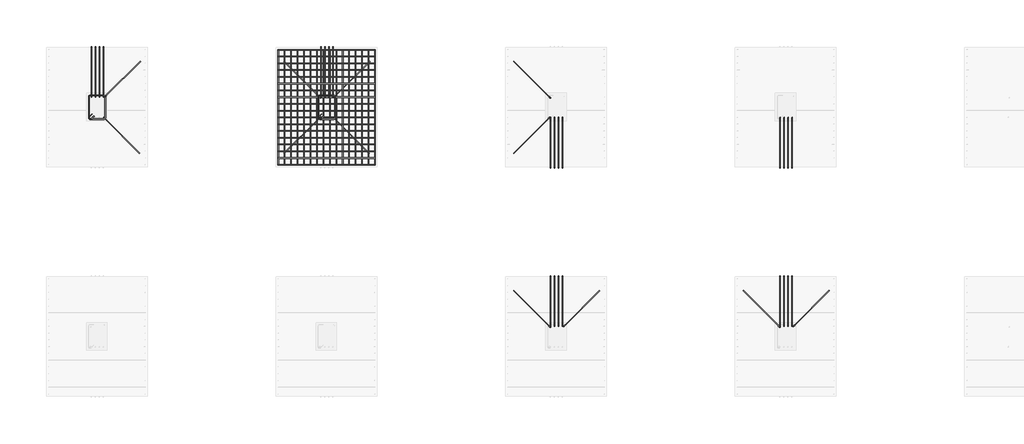
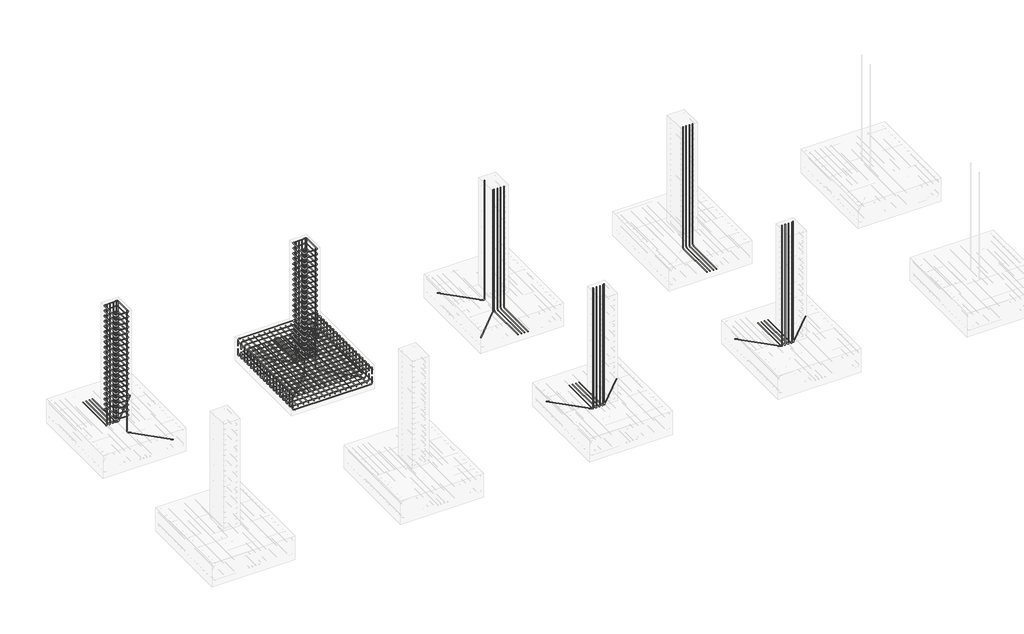
# One storey, part 9 of 33: 24 reinforcing bars.
"""IFC4 building model written with IfcOpenShell, lengths in millimetres."""

from ifc_helpers import new_model, si_unit, point, frame, origin, place, context, project, spatial, polyline, circle_curve, trimmed, segment, composite_curve, source, transform, mapped, element, save
from ifc_brep_helpers import swept_disk

model = new_model("IFC4")

# Units and contexts
model_context = context("Model", 3, world=origin())
ifc_project = project(units=[si_unit("LENGTHUNIT", "METRE", prefix="MILLI")], contexts=[model_context])

# Site, building, storey
site = spatial("IfcSite", under=ifc_project)
building = spatial("IfcBuilding", under=site)
storey = spatial("IfcBuildingStorey", under=building, Elevation=-3000.0)

# Reinforcing bars
placement = place(None, origin())
reinforcing_bar_shape = source(origin(), model_context, "Body", "SolidModel", [
    swept_disk(composite_curve([segment(polyline([(4306.5357258, -2044.0608134, -3240.0), (4306.5357258, -2044.0608134, -3092.7)]), True, "CONTINUOUS"), segment(trimmed(circle_curve(frame((4352.8857258, -2044.0608134, -3092.7), z_axis=(0.0, 1.0, 0.0), x_axis=(-46.349999999999454, 0.0, 0.0)), 46.35), [point((4306.5357258, -2044.0608134, -3092.7))], [point((4352.8857258, -2044.0608134, -3046.35))], True, "CARTESIAN"), True, "CONTINUOUS"), segment(polyline([(4352.8857258, -2044.0608134, -3046.35), (6367.4857258, -2044.0608134, -3046.35)]), True, "CONTINUOUS"), segment(trimmed(circle_curve(frame((6367.4857258, -2044.0608134, -3092.7), z_axis=(0.0, 1.0, 0.0), x_axis=(0.0, 0.0, 46.34999999999991)), 46.35), [point((6367.4857258, -2044.0608134, -3046.35))], [point((6413.8357258, -2044.0608134, -3092.7))], True, "CARTESIAN"), True, "CONTINUOUS"), segment(polyline([(6413.8357258, -2044.0608134, -3092.7), (6413.8357258, -2044.0608134, -3240.0)]), True, "CONTINUOUS")], self_intersect=False), 6.35),
])
element("IfcReinforcingBar", 1, at=placement, inside=storey, context=model_context, shape_type="MappedRepresentation", body=[
    mapped(reinforcing_bar_shape, transform((0.0, 0.0, 0.0), x_axis=(1.0, 0.0, 0.0), y_axis=(0.0, 1.0, 0.0), z_axis=(0.0, 0.0, 1.0))),
    mapped(reinforcing_bar_shape, transform((0.0, -147.4882353, 0.0), x_axis=(1.0, 0.0, 0.0), y_axis=(0.0, 1.0, 0.0), z_axis=(0.0, 0.0, 1.0))),
    mapped(reinforcing_bar_shape, transform((0.0, -294.9764706, 0.0), x_axis=(1.0, 0.0, 0.0), y_axis=(0.0, 1.0, 0.0), z_axis=(0.0, 0.0, 1.0))),
    mapped(reinforcing_bar_shape, transform((0.0, -442.4647059, 0.0), x_axis=(1.0, 0.0, 0.0), y_axis=(0.0, 1.0, 0.0), z_axis=(0.0, 0.0, 1.0))),
    mapped(reinforcing_bar_shape, transform((0.0, -589.9529412, 0.0), x_axis=(1.0, 0.0, 0.0), y_axis=(0.0, 1.0, 0.0), z_axis=(0.0, 0.0, 1.0))),
    mapped(reinforcing_bar_shape, transform((0.0, -737.4411765, 0.0), x_axis=(1.0, 0.0, 0.0), y_axis=(0.0, 1.0, 0.0), z_axis=(0.0, 0.0, 1.0))),
    mapped(reinforcing_bar_shape, transform((0.0, -884.9294118, 0.0), x_axis=(1.0, 0.0, 0.0), y_axis=(0.0, 1.0, 0.0), z_axis=(0.0, 0.0, 1.0))),
    mapped(reinforcing_bar_shape, transform((0.0, -1032.4176471, 0.0), x_axis=(1.0, 0.0, 0.0), y_axis=(0.0, 1.0, 0.0), z_axis=(0.0, 0.0, 1.0))),
    mapped(reinforcing_bar_shape, transform((0.0, -1179.9058824, 0.0), x_axis=(1.0, 0.0, 0.0), y_axis=(0.0, 1.0, 0.0), z_axis=(0.0, 0.0, 1.0))),
    mapped(reinforcing_bar_shape, transform((0.0, -1327.3941176, 0.0), x_axis=(1.0, 0.0, 0.0), y_axis=(0.0, 1.0, 0.0), z_axis=(0.0, 0.0, 1.0))),
    mapped(reinforcing_bar_shape, transform((0.0, -1474.8823529, 0.0), x_axis=(1.0, 0.0, 0.0), y_axis=(0.0, 1.0, 0.0), z_axis=(0.0, 0.0, 1.0))),
    mapped(reinforcing_bar_shape, transform((0.0, -1622.3705882, 0.0), x_axis=(1.0, 0.0, 0.0), y_axis=(0.0, 1.0, 0.0), z_axis=(0.0, 0.0, 1.0))),
    mapped(reinforcing_bar_shape, transform((0.0, -1769.8588235, 0.0), x_axis=(1.0, 0.0, 0.0), y_axis=(0.0, 1.0, 0.0), z_axis=(0.0, 0.0, 1.0))),
    mapped(reinforcing_bar_shape, transform((0.0, -1917.3470588, 0.0), x_axis=(1.0, 0.0, 0.0), y_axis=(0.0, 1.0, 0.0), z_axis=(0.0, 0.0, 1.0))),
    mapped(reinforcing_bar_shape, transform((0.0, -2064.8352941, 0.0), x_axis=(1.0, 0.0, 0.0), y_axis=(0.0, 1.0, 0.0), z_axis=(0.0, 0.0, 1.0))),
    mapped(reinforcing_bar_shape, transform((0.0, -2212.3235294, 0.0), x_axis=(1.0, 0.0, 0.0), y_axis=(0.0, 1.0, 0.0), z_axis=(0.0, 0.0, 1.0))),
    mapped(reinforcing_bar_shape, transform((0.0, -2359.8117647, 0.0), x_axis=(1.0, 0.0, 0.0), y_axis=(0.0, 1.0, 0.0), z_axis=(0.0, 0.0, 1.0))),
    mapped(reinforcing_bar_shape, transform((0.0, -2507.3, 0.0), x_axis=(1.0, 0.0, 0.0), y_axis=(0.0, 1.0, 0.0), z_axis=(0.0, 0.0, 1.0))),
])
reinforcing_bar_2_shape = source(origin(), model_context, "Body", "SolidModel", [
    swept_disk(composite_curve([segment(polyline([(6413.8357258, -2044.0608134, -3330.080452), (6413.8357258, -2044.0608134, -3477.380452)]), True, "CONTINUOUS"), segment(trimmed(circle_curve(frame((6367.4857258, -2044.0608134, -3477.380452), z_axis=(0.0, 1.0, 0.0), x_axis=(46.349999999999454, 0.0, 0.0)), 46.35), [point((6413.8357258, -2044.0608134, -3477.380452))], [point((6367.4857258, -2044.0608134, -3523.730452))], True, "CARTESIAN"), True, "CONTINUOUS"), segment(polyline([(6367.4857258, -2044.0608134, -3523.730452), (4352.8857258, -2044.0608134, -3523.730452)]), True, "CONTINUOUS"), segment(trimmed(circle_curve(frame((4352.8857258, -2044.0608134, -3477.380452), z_axis=(0.0, 1.0, 0.0), x_axis=(0.0, 0.0, -46.34999999999991)), 46.35), [point((4352.8857258, -2044.0608134, -3523.730452))], [point((4306.5357258, -2044.0608134, -3477.380452))], True, "CARTESIAN"), True, "CONTINUOUS"), segment(polyline([(4306.5357258, -2044.0608134, -3477.380452), (4306.5357258, -2044.0608134, -3330.080452)]), True, "CONTINUOUS")], self_intersect=False), 6.35),
])
element("IfcReinforcingBar", 2, at=placement, inside=storey, context=model_context, shape_type="MappedRepresentation", body=[
    mapped(reinforcing_bar_2_shape, transform((0.0, 0.0, 0.0), x_axis=(1.0, 0.0, 0.0), y_axis=(0.0, 1.0, 0.0), z_axis=(0.0, 0.0, 1.0))),
    mapped(reinforcing_bar_2_shape, transform((0.0, -147.4882353, 0.0), x_axis=(1.0, 0.0, 0.0), y_axis=(0.0, 1.0, 0.0), z_axis=(0.0, 0.0, 1.0))),
    mapped(reinforcing_bar_2_shape, transform((0.0, -294.9764706, 0.0), x_axis=(1.0, 0.0, 0.0), y_axis=(0.0, 1.0, 0.0), z_axis=(0.0, 0.0, 1.0))),
    mapped(reinforcing_bar_2_shape, transform((0.0, -442.4647059, 0.0), x_axis=(1.0, 0.0, 0.0), y_axis=(0.0, 1.0, 0.0), z_axis=(0.0, 0.0, 1.0))),
    mapped(reinforcing_bar_2_shape, transform((0.0, -589.9529412, 0.0), x_axis=(1.0, 0.0, 0.0), y_axis=(0.0, 1.0, 0.0), z_axis=(0.0, 0.0, 1.0))),
    mapped(reinforcing_bar_2_shape, transform((0.0, -737.4411765, 0.0), x_axis=(1.0, 0.0, 0.0), y_axis=(0.0, 1.0, 0.0), z_axis=(0.0, 0.0, 1.0))),
    mapped(reinforcing_bar_2_shape, transform((0.0, -884.9294118, 0.0), x_axis=(1.0, 0.0, 0.0), y_axis=(0.0, 1.0, 0.0), z_axis=(0.0, 0.0, 1.0))),
    mapped(reinforcing_bar_2_shape, transform((0.0, -1032.4176471, 0.0), x_axis=(1.0, 0.0, 0.0), y_axis=(0.0, 1.0, 0.0), z_axis=(0.0, 0.0, 1.0))),
    mapped(reinforcing_bar_2_shape, transform((0.0, -1179.9058824, 0.0), x_axis=(1.0, 0.0, 0.0), y_axis=(0.0, 1.0, 0.0), z_axis=(0.0, 0.0, 1.0))),
    mapped(reinforcing_bar_2_shape, transform((0.0, -1327.3941176, 0.0), x_axis=(1.0, 0.0, 0.0), y_axis=(0.0, 1.0, 0.0), z_axis=(0.0, 0.0, 1.0))),
    mapped(reinforcing_bar_2_shape, transform((0.0, -1474.8823529, 0.0), x_axis=(1.0, 0.0, 0.0), y_axis=(0.0, 1.0, 0.0), z_axis=(0.0, 0.0, 1.0))),
    mapped(reinforcing_bar_2_shape, transform((0.0, -1622.3705882, 0.0), x_axis=(1.0, 0.0, 0.0), y_axis=(0.0, 1.0, 0.0), z_axis=(0.0, 0.0, 1.0))),
    mapped(reinforcing_bar_2_shape, transform((0.0, -1769.8588235, 0.0), x_axis=(1.0, 0.0, 0.0), y_axis=(0.0, 1.0, 0.0), z_axis=(0.0, 0.0, 1.0))),
    mapped(reinforcing_bar_2_shape, transform((0.0, -1917.3470588, 0.0), x_axis=(1.0, 0.0, 0.0), y_axis=(0.0, 1.0, 0.0), z_axis=(0.0, 0.0, 1.0))),
    mapped(reinforcing_bar_2_shape, transform((0.0, -2064.8352941, 0.0), x_axis=(1.0, 0.0, 0.0), y_axis=(0.0, 1.0, 0.0), z_axis=(0.0, 0.0, 1.0))),
    mapped(reinforcing_bar_2_shape, transform((0.0, -2212.3235294, 0.0), x_axis=(1.0, 0.0, 0.0), y_axis=(0.0, 1.0, 0.0), z_axis=(0.0, 0.0, 1.0))),
    mapped(reinforcing_bar_2_shape, transform((0.0, -2359.8117647, 0.0), x_axis=(1.0, 0.0, 0.0), y_axis=(0.0, 1.0, 0.0), z_axis=(0.0, 0.0, 1.0))),
    mapped(reinforcing_bar_2_shape, transform((0.0, -2507.3, 0.0), x_axis=(1.0, 0.0, 0.0), y_axis=(0.0, 1.0, 0.0), z_axis=(0.0, 0.0, 1.0))),
])
reinforcing_bar_3_shape = source(origin(), model_context, "Body", "SolidModel", [
    swept_disk(composite_curve([segment(polyline([(6413.8357258, -4557.7108134, -3447.8614173), (6413.8357258, -2037.7108134, -3447.8614173)]), True, "CONTINUOUS")], self_intersect=False), 6.35),
])
element("IfcReinforcingBar", 3, at=placement, inside=storey, context=model_context, shape_type="MappedRepresentation", body=[
    mapped(reinforcing_bar_3_shape, transform((0.0, 0.0, 0.0), x_axis=(1.0, 0.0, 0.0), y_axis=(0.0, 1.0, 0.0), z_axis=(0.0, 0.0, 1.0))),
    mapped(reinforcing_bar_3_shape, transform((-140.4866667, 0.0, 0.0), x_axis=(1.0, 0.0, 0.0), y_axis=(0.0, 1.0, 0.0), z_axis=(0.0, 0.0, 1.0))),
    mapped(reinforcing_bar_3_shape, transform((-280.9733333, 0.0, 0.0), x_axis=(1.0, 0.0, 0.0), y_axis=(0.0, 1.0, 0.0), z_axis=(0.0, 0.0, 1.0))),
    mapped(reinforcing_bar_3_shape, transform((-421.46, 0.0, 0.0), x_axis=(1.0, 0.0, 0.0), y_axis=(0.0, 1.0, 0.0), z_axis=(0.0, 0.0, 1.0))),
    mapped(reinforcing_bar_3_shape, transform((-561.9466667, 0.0, 0.0), x_axis=(1.0, 0.0, 0.0), y_axis=(0.0, 1.0, 0.0), z_axis=(0.0, 0.0, 1.0))),
    mapped(reinforcing_bar_3_shape, transform((-702.4333333, 0.0, 0.0), x_axis=(1.0, 0.0, 0.0), y_axis=(0.0, 1.0, 0.0), z_axis=(0.0, 0.0, 1.0))),
    mapped(reinforcing_bar_3_shape, transform((-842.92, 0.0, 0.0), x_axis=(1.0, 0.0, 0.0), y_axis=(0.0, 1.0, 0.0), z_axis=(0.0, 0.0, 1.0))),
    mapped(reinforcing_bar_3_shape, transform((-983.4066667, 0.0, 0.0), x_axis=(1.0, 0.0, 0.0), y_axis=(0.0, 1.0, 0.0), z_axis=(0.0, 0.0, 1.0))),
    mapped(reinforcing_bar_3_shape, transform((-1123.8933333, 0.0, 0.0), x_axis=(1.0, 0.0, 0.0), y_axis=(0.0, 1.0, 0.0), z_axis=(0.0, 0.0, 1.0))),
    mapped(reinforcing_bar_3_shape, transform((-1264.38, 0.0, 0.0), x_axis=(1.0, 0.0, 0.0), y_axis=(0.0, 1.0, 0.0), z_axis=(0.0, 0.0, 1.0))),
    mapped(reinforcing_bar_3_shape, transform((-1404.8666667, 0.0, 0.0), x_axis=(1.0, 0.0, 0.0), y_axis=(0.0, 1.0, 0.0), z_axis=(0.0, 0.0, 1.0))),
    mapped(reinforcing_bar_3_shape, transform((-1545.3533333, 0.0, 0.0), x_axis=(1.0, 0.0, 0.0), y_axis=(0.0, 1.0, 0.0), z_axis=(0.0, 0.0, 1.0))),
    mapped(reinforcing_bar_3_shape, transform((-1685.84, 0.0, 0.0), x_axis=(1.0, 0.0, 0.0), y_axis=(0.0, 1.0, 0.0), z_axis=(0.0, 0.0, 1.0))),
    mapped(reinforcing_bar_3_shape, transform((-1826.3266667, 0.0, 0.0), x_axis=(1.0, 0.0, 0.0), y_axis=(0.0, 1.0, 0.0), z_axis=(0.0, 0.0, 1.0))),
    mapped(reinforcing_bar_3_shape, transform((-1966.8133333, 0.0, 0.0), x_axis=(1.0, 0.0, 0.0), y_axis=(0.0, 1.0, 0.0), z_axis=(0.0, 0.0, 1.0))),
    mapped(reinforcing_bar_3_shape, transform((-2107.3, 0.0, 0.0), x_axis=(1.0, 0.0, 0.0), y_axis=(0.0, 1.0, 0.0), z_axis=(0.0, 0.0, 1.0))),
])
reinforcing_bar_4_shape = source(origin(), model_context, "Body", "SolidModel", [
    swept_disk(composite_curve([segment(polyline([(4306.5357258, -4557.7108134, -3122.7084113), (4306.5357258, -2037.7108134, -3122.7084113)]), True, "CONTINUOUS")], self_intersect=False), 6.35),
])
element("IfcReinforcingBar", 4, at=placement, inside=storey, context=model_context, shape_type="MappedRepresentation", body=[
    mapped(reinforcing_bar_4_shape, transform((0.0, 0.0, 0.0), x_axis=(1.0, 0.0, 0.0), y_axis=(0.0, 1.0, 0.0), z_axis=(0.0, 0.0, 1.0))),
    mapped(reinforcing_bar_4_shape, transform((140.4866667, 0.0, 0.0), x_axis=(1.0, 0.0, 0.0), y_axis=(0.0, 1.0, 0.0), z_axis=(0.0, 0.0, 1.0))),
    mapped(reinforcing_bar_4_shape, transform((280.9733333, 0.0, 0.0), x_axis=(1.0, 0.0, 0.0), y_axis=(0.0, 1.0, 0.0), z_axis=(0.0, 0.0, 1.0))),
    mapped(reinforcing_bar_4_shape, transform((421.46, 0.0, 0.0), x_axis=(1.0, 0.0, 0.0), y_axis=(0.0, 1.0, 0.0), z_axis=(0.0, 0.0, 1.0))),
    mapped(reinforcing_bar_4_shape, transform((561.9466667, 0.0, 0.0), x_axis=(1.0, 0.0, 0.0), y_axis=(0.0, 1.0, 0.0), z_axis=(0.0, 0.0, 1.0))),
    mapped(reinforcing_bar_4_shape, transform((702.4333333, 0.0, 0.0), x_axis=(1.0, 0.0, 0.0), y_axis=(0.0, 1.0, 0.0), z_axis=(0.0, 0.0, 1.0))),
    mapped(reinforcing_bar_4_shape, transform((842.92, 0.0, 0.0), x_axis=(1.0, 0.0, 0.0), y_axis=(0.0, 1.0, 0.0), z_axis=(0.0, 0.0, 1.0))),
    mapped(reinforcing_bar_4_shape, transform((983.4066667, 0.0, 0.0), x_axis=(1.0, 0.0, 0.0), y_axis=(0.0, 1.0, 0.0), z_axis=(0.0, 0.0, 1.0))),
    mapped(reinforcing_bar_4_shape, transform((1123.8933333, 0.0, 0.0), x_axis=(1.0, 0.0, 0.0), y_axis=(0.0, 1.0, 0.0), z_axis=(0.0, 0.0, 1.0))),
    mapped(reinforcing_bar_4_shape, transform((1264.38, 0.0, 0.0), x_axis=(1.0, 0.0, 0.0), y_axis=(0.0, 1.0, 0.0), z_axis=(0.0, 0.0, 1.0))),
    mapped(reinforcing_bar_4_shape, transform((1404.8666667, 0.0, 0.0), x_axis=(1.0, 0.0, 0.0), y_axis=(0.0, 1.0, 0.0), z_axis=(0.0, 0.0, 1.0))),
    mapped(reinforcing_bar_4_shape, transform((1545.3533333, 0.0, 0.0), x_axis=(1.0, 0.0, 0.0), y_axis=(0.0, 1.0, 0.0), z_axis=(0.0, 0.0, 1.0))),
    mapped(reinforcing_bar_4_shape, transform((1685.84, 0.0, 0.0), x_axis=(1.0, 0.0, 0.0), y_axis=(0.0, 1.0, 0.0), z_axis=(0.0, 0.0, 1.0))),
    mapped(reinforcing_bar_4_shape, transform((1826.3266667, 0.0, 0.0), x_axis=(1.0, 0.0, 0.0), y_axis=(0.0, 1.0, 0.0), z_axis=(0.0, 0.0, 1.0))),
    mapped(reinforcing_bar_4_shape, transform((1966.8133333, 0.0, 0.0), x_axis=(1.0, 0.0, 0.0), y_axis=(0.0, 1.0, 0.0), z_axis=(0.0, 0.0, 1.0))),
    mapped(reinforcing_bar_4_shape, transform((2107.3, 0.0, 0.0), x_axis=(1.0, 0.0, 0.0), y_axis=(0.0, 1.0, 0.0), z_axis=(0.0, 0.0, 1.0))),
])
reinforcing_bar_5_shape = source(origin(), model_context, "Body", "SolidModel", [
    swept_disk(composite_curve([segment(polyline([(246.4614911, -3446.8994528, -2953.65), (190.7179282, -3502.6430158, -2953.65)]), True, "CONTINUOUS"), segment(trimmed(circle_curve(frame((212.8857258, -3524.8108134, -2953.65), z_axis=(0.0, 0.0, 1.0), x_axis=(-22.1677976, 22.167797600000085, 0.0)), 31.35), [point((190.7179282, -3502.6430158, -2953.65))], [point((212.8857258, -3556.1608134, -2953.65))], True, "CARTESIAN"), True, "CONTINUOUS"), segment(polyline([(212.8857258, -3556.1608134, -2953.65), (507.4857258, -3556.1608134, -2953.65)]), True, "CONTINUOUS"), segment(trimmed(circle_curve(frame((507.4857258, -3524.8108134, -2953.65), z_axis=(0.0, 0.0, 1.0), x_axis=(0.0, -31.34999999999991, 0.0)), 31.35), [point((507.4857258, -3556.1608134, -2953.65))], [point((538.8357258, -3524.8108134, -2953.65))], True, "CARTESIAN"), True, "CONTINUOUS"), segment(polyline([(538.8357258, -3524.8108134, -2953.65), (538.8357258, -3070.6108134, -2953.65)]), True, "CONTINUOUS"), segment(trimmed(circle_curve(frame((507.5055109, -3070.6108134, -2954.7636125), z_axis=(-0.0355219283344822, 0.0, 0.9993688971583016), x_axis=(31.330214899999987, 0.0, 1.1136124999998174)), 31.35), [point((538.8357258, -3070.6108134, -2953.65))], [point((507.5055109, -3039.2608134, -2954.7636125))], True, "CARTESIAN"), True, "CONTINUOUS"), segment(polyline([(507.5055109, -3039.2608134, -2954.7636125), (212.8659407, -3039.2608134, -2965.2363875)]), True, "CONTINUOUS"), segment(trimmed(circle_curve(frame((212.8659407, -3070.6108134, -2965.2363875), z_axis=(-0.0355219283344822, 0.0, 0.9993688971583016), x_axis=(0.0, 31.34999999999991, 0.0)), 31.35), [point((212.8659407, -3039.2608134, -2965.2363875))], [point((181.5357258, -3070.6108134, -2966.35))], True, "CARTESIAN"), True, "CONTINUOUS"), segment(polyline([(181.5357258, -3070.6108134, -2966.35), (181.5357258, -3524.8108134, -2966.35)]), True, "CONTINUOUS"), segment(trimmed(circle_curve(frame((212.8857258, -3524.8108134, -2966.35), z_axis=(0.0, 0.0, 1.0), x_axis=(-31.349999999999994, 0.0, 0.0)), 31.35), [point((181.5357258, -3524.8108134, -2966.35))], [point((235.0535234, -3546.978611, -2966.35))], True, "CARTESIAN"), True, "CONTINUOUS"), segment(polyline([(235.0535234, -3546.978611, -2966.35), (290.7970863, -3491.235048, -2966.35)]), True, "CONTINUOUS")], self_intersect=False), 6.35),
])
element("IfcReinforcingBar", 5, at=placement, inside=storey, context=model_context, shape_type="MappedRepresentation", body=[
    mapped(reinforcing_bar_5_shape, transform((0.0, 0.0, 0.0), x_axis=(1.0, 0.0, 0.0), y_axis=(0.0, 1.0, 0.0), z_axis=(0.0, 0.0, 1.0))),
    mapped(reinforcing_bar_5_shape, transform((0.0, 0.0, 145.365), x_axis=(1.0, 0.0, 0.0), y_axis=(0.0, 1.0, 0.0), z_axis=(0.0, 0.0, 1.0))),
    mapped(reinforcing_bar_5_shape, transform((0.0, 0.0, 290.73), x_axis=(1.0, 0.0, 0.0), y_axis=(0.0, 1.0, 0.0), z_axis=(0.0, 0.0, 1.0))),
    mapped(reinforcing_bar_5_shape, transform((0.0, 0.0, 436.095), x_axis=(1.0, 0.0, 0.0), y_axis=(0.0, 1.0, 0.0), z_axis=(0.0, 0.0, 1.0))),
    mapped(reinforcing_bar_5_shape, transform((0.0, 0.0, 581.46), x_axis=(1.0, 0.0, 0.0), y_axis=(0.0, 1.0, 0.0), z_axis=(0.0, 0.0, 1.0))),
    mapped(reinforcing_bar_5_shape, transform((0.0, 0.0, 726.825), x_axis=(1.0, 0.0, 0.0), y_axis=(0.0, 1.0, 0.0), z_axis=(0.0, 0.0, 1.0))),
    mapped(reinforcing_bar_5_shape, transform((0.0, 0.0, 872.19), x_axis=(1.0, 0.0, 0.0), y_axis=(0.0, 1.0, 0.0), z_axis=(0.0, 0.0, 1.0))),
    mapped(reinforcing_bar_5_shape, transform((0.0, 0.0, 1017.555), x_axis=(1.0, 0.0, 0.0), y_axis=(0.0, 1.0, 0.0), z_axis=(0.0, 0.0, 1.0))),
    mapped(reinforcing_bar_5_shape, transform((0.0, 0.0, 1162.92), x_axis=(1.0, 0.0, 0.0), y_axis=(0.0, 1.0, 0.0), z_axis=(0.0, 0.0, 1.0))),
    mapped(reinforcing_bar_5_shape, transform((0.0, 0.0, 1308.285), x_axis=(1.0, 0.0, 0.0), y_axis=(0.0, 1.0, 0.0), z_axis=(0.0, 0.0, 1.0))),
    mapped(reinforcing_bar_5_shape, transform((0.0, 0.0, 1453.65), x_axis=(1.0, 0.0, 0.0), y_axis=(0.0, 1.0, 0.0), z_axis=(0.0, 0.0, 1.0))),
    mapped(reinforcing_bar_5_shape, transform((0.0, 0.0, 1599.015), x_axis=(1.0, 0.0, 0.0), y_axis=(0.0, 1.0, 0.0), z_axis=(0.0, 0.0, 1.0))),
    mapped(reinforcing_bar_5_shape, transform((0.0, 0.0, 1744.38), x_axis=(1.0, 0.0, 0.0), y_axis=(0.0, 1.0, 0.0), z_axis=(0.0, 0.0, 1.0))),
    mapped(reinforcing_bar_5_shape, transform((0.0, 0.0, 1889.745), x_axis=(1.0, 0.0, 0.0), y_axis=(0.0, 1.0, 0.0), z_axis=(0.0, 0.0, 1.0))),
    mapped(reinforcing_bar_5_shape, transform((0.0, 0.0, 2035.11), x_axis=(1.0, 0.0, 0.0), y_axis=(0.0, 1.0, 0.0), z_axis=(0.0, 0.0, 1.0))),
    mapped(reinforcing_bar_5_shape, transform((0.0, 0.0, 2180.475), x_axis=(1.0, 0.0, 0.0), y_axis=(0.0, 1.0, 0.0), z_axis=(0.0, 0.0, 1.0))),
    mapped(reinforcing_bar_5_shape, transform((0.0, 0.0, 2325.84), x_axis=(1.0, 0.0, 0.0), y_axis=(0.0, 1.0, 0.0), z_axis=(0.0, 0.0, 1.0))),
    mapped(reinforcing_bar_5_shape, transform((0.0, 0.0, 2471.205), x_axis=(1.0, 0.0, 0.0), y_axis=(0.0, 1.0, 0.0), z_axis=(0.0, 0.0, 1.0))),
    mapped(reinforcing_bar_5_shape, transform((0.0, 0.0, 2616.57), x_axis=(1.0, 0.0, 0.0), y_axis=(0.0, 1.0, 0.0), z_axis=(0.0, 0.0, 1.0))),
    mapped(reinforcing_bar_5_shape, transform((0.0, 0.0, 2761.935), x_axis=(1.0, 0.0, 0.0), y_axis=(0.0, 1.0, 0.0), z_axis=(0.0, 0.0, 1.0))),
    mapped(reinforcing_bar_5_shape, transform((0.0, 0.0, 2907.3), x_axis=(1.0, 0.0, 0.0), y_axis=(0.0, 1.0, 0.0), z_axis=(0.0, 0.0, 1.0))),
])
element("IfcReinforcingBar", 6, at=placement, inside=storey, context=model_context, shape_type="SolidModel", body=[
    swept_disk(composite_curve([segment(polyline([(507.1671301, -3521.6339414, -40.0), (507.1671301, -3521.6339414, -3393.65)]), True, "CONTINUOUS"), segment(trimmed(circle_curve(frame((539.9415294, -3554.4083407, -3393.65), z_axis=(-0.7071067811865493, -0.7071067811865459, 0.0), x_axis=(-32.77439930000003, 32.774399299999914, 0.0)), 46.35), [point((507.1671301, -3521.6339414, -3393.65))], [point((539.9415294, -3554.4083407, -3440.0))], True, "CARTESIAN"), True, "CONTINUOUS"), segment(polyline([(539.9415294, -3554.4083407, -3440.0), (1284.9845894, -4299.4514007, -3440.0)]), True, "CONTINUOUS")], self_intersect=False), 6.35),
])
element("IfcReinforcingBar", 7, at=placement, inside=storey, context=model_context, shape_type="SolidModel", body=[
    swept_disk(composite_curve([segment(polyline([(525.7684217, -3073.7876853, -30.2564663), (525.7684217, -3073.7876853, -3383.9064663)]), True, "CONTINUOUS"), segment(trimmed(circle_curve(frame((558.542821, -3041.013286, -3383.9064663), z_axis=(0.7071067811865493, -0.7071067811865459, 0.0), x_axis=(-32.77439930000003, -32.774399299999914, 0.0)), 46.35), [point((525.7684217, -3073.7876853, -3383.9064663))], [point((558.542821, -3041.013286, -3430.2564663))], True, "CARTESIAN"), True, "CONTINUOUS"), segment(polyline([(558.542821, -3041.013286, -3430.2564663), (1303.585881, -2295.970226, -3430.2564663)]), True, "CONTINUOUS")], self_intersect=False), 6.35),
])
reinforcing_bar_6_shape = source(origin(), model_context, "Body", "SolidModel", [
    swept_disk(composite_curve([segment(polyline([(236.1158322, -3071.9278134, -40.0), (236.1158322, -3071.9278134, -3393.65)]), True, "CONTINUOUS"), segment(trimmed(circle_curve(frame((236.1158322, -3025.5778134, -3393.65), z_axis=(1.0, 0.0, 0.0), x_axis=(0.0, -46.34999999999991, 0.0)), 46.35), [point((236.1158322, -3071.9278134, -3393.65))], [point((236.1158322, -3025.5778134, -3440.0))], True, "CARTESIAN"), True, "CONTINUOUS"), segment(polyline([(236.1158322, -3025.5778134, -3440.0), (236.1158322, -1971.9278134, -3440.0)]), True, "CONTINUOUS")], self_intersect=False), 6.35),
])
element("IfcReinforcingBar", 8, at=placement, inside=storey, context=model_context, shape_type="MappedRepresentation", body=[
    mapped(reinforcing_bar_6_shape, transform((0.0, 0.0, 0.0), x_axis=(1.0, 0.0, 0.0), y_axis=(0.0, 1.0, 0.0), z_axis=(0.0, 0.0, 1.0))),
    mapped(reinforcing_bar_6_shape, transform((86.8979716, 0.0, 0.0), x_axis=(1.0, 0.0, 0.0), y_axis=(0.0, 1.0, 0.0), z_axis=(0.0, 0.0, 1.0))),
    mapped(reinforcing_bar_6_shape, transform((173.7959432, 0.0, 0.0), x_axis=(1.0, 0.0, 0.0), y_axis=(0.0, 1.0, 0.0), z_axis=(0.0, 0.0, 1.0))),
    mapped(reinforcing_bar_6_shape, transform((260.6939148, 0.0, 0.0), x_axis=(1.0, 0.0, 0.0), y_axis=(0.0, 1.0, 0.0), z_axis=(0.0, 0.0, 1.0))),
])
reinforcing_bar_7_shape = source(origin(), model_context, "Body", "SolidModel", [
    swept_disk(composite_curve([segment(polyline([(5246.4614911, -3446.8994528, -2953.65), (5190.7179282, -3502.6430158, -2953.65)]), True, "CONTINUOUS"), segment(trimmed(circle_curve(frame((5212.8857258, -3524.8108134, -2953.65), z_axis=(0.0, 0.0, 1.0), x_axis=(-22.167797600000085, 22.167797600000085, 0.0)), 31.35), [point((5190.7179282, -3502.6430158, -2953.65))], [point((5212.8857258, -3556.1608134, -2953.65))], True, "CARTESIAN"), True, "CONTINUOUS"), segment(polyline([(5212.8857258, -3556.1608134, -2953.65), (5507.4857258, -3556.1608134, -2953.65)]), True, "CONTINUOUS"), segment(trimmed(circle_curve(frame((5507.4857258, -3524.8108134, -2953.65), z_axis=(0.0, 0.0, 1.0), x_axis=(0.0, -31.34999999999991, 0.0)), 31.35), [point((5507.4857258, -3556.1608134, -2953.65))], [point((5538.8357258, -3524.8108134, -2953.65))], True, "CARTESIAN"), True, "CONTINUOUS"), segment(polyline([(5538.8357258, -3524.8108134, -2953.65), (5538.8357258, -3070.6108134, -2953.65)]), True, "CONTINUOUS"), segment(trimmed(circle_curve(frame((5507.5055109, -3070.6108134, -2954.7636125), z_axis=(-0.0355219283344822, 0.0, 0.9993688971583016), x_axis=(31.33021489999919, 0.0, 1.1136124999998174)), 31.35), [point((5538.8357258, -3070.6108134, -2953.65))], [point((5507.5055109, -3039.2608134, -2954.7636125))], True, "CARTESIAN"), True, "CONTINUOUS"), segment(polyline([(5507.5055109, -3039.2608134, -2954.7636125), (5212.8659407, -3039.2608134, -2965.2363875)]), True, "CONTINUOUS"), segment(trimmed(circle_curve(frame((5212.8659407, -3070.6108134, -2965.2363875), z_axis=(-0.0355219283344822, 0.0, 0.9993688971583016), x_axis=(0.0, 31.34999999999991, 0.0)), 31.35), [point((5212.8659407, -3039.2608134, -2965.2363875))], [point((5181.5357258, -3070.6108134, -2966.35))], True, "CARTESIAN"), True, "CONTINUOUS"), segment(polyline([(5181.5357258, -3070.6108134, -2966.35), (5181.5357258, -3524.8108134, -2966.35)]), True, "CONTINUOUS"), segment(trimmed(circle_curve(frame((5212.8857258, -3524.8108134, -2966.35), z_axis=(0.0, 0.0, 1.0), x_axis=(-31.349999999999454, 0.0, 0.0)), 31.35), [point((5181.5357258, -3524.8108134, -2966.35))], [point((5235.0535234, -3546.978611, -2966.35))], True, "CARTESIAN"), True, "CONTINUOUS"), segment(polyline([(5235.0535234, -3546.978611, -2966.35), (5290.7970863, -3491.235048, -2966.35)]), True, "CONTINUOUS")], self_intersect=False), 6.35),
])
element("IfcReinforcingBar", 9, at=placement, inside=storey, context=model_context, shape_type="MappedRepresentation", body=[
    mapped(reinforcing_bar_7_shape, transform((0.0, 0.0, 0.0), x_axis=(1.0, 0.0, 0.0), y_axis=(0.0, 1.0, 0.0), z_axis=(0.0, 0.0, 1.0))),
    mapped(reinforcing_bar_7_shape, transform((0.0, 0.0, 145.365), x_axis=(1.0, 0.0, 0.0), y_axis=(0.0, 1.0, 0.0), z_axis=(0.0, 0.0, 1.0))),
    mapped(reinforcing_bar_7_shape, transform((0.0, 0.0, 290.73), x_axis=(1.0, 0.0, 0.0), y_axis=(0.0, 1.0, 0.0), z_axis=(0.0, 0.0, 1.0))),
    mapped(reinforcing_bar_7_shape, transform((0.0, 0.0, 436.095), x_axis=(1.0, 0.0, 0.0), y_axis=(0.0, 1.0, 0.0), z_axis=(0.0, 0.0, 1.0))),
    mapped(reinforcing_bar_7_shape, transform((0.0, 0.0, 581.46), x_axis=(1.0, 0.0, 0.0), y_axis=(0.0, 1.0, 0.0), z_axis=(0.0, 0.0, 1.0))),
    mapped(reinforcing_bar_7_shape, transform((0.0, 0.0, 726.825), x_axis=(1.0, 0.0, 0.0), y_axis=(0.0, 1.0, 0.0), z_axis=(0.0, 0.0, 1.0))),
    mapped(reinforcing_bar_7_shape, transform((0.0, 0.0, 872.19), x_axis=(1.0, 0.0, 0.0), y_axis=(0.0, 1.0, 0.0), z_axis=(0.0, 0.0, 1.0))),
    mapped(reinforcing_bar_7_shape, transform((0.0, 0.0, 1017.555), x_axis=(1.0, 0.0, 0.0), y_axis=(0.0, 1.0, 0.0), z_axis=(0.0, 0.0, 1.0))),
    mapped(reinforcing_bar_7_shape, transform((0.0, 0.0, 1162.92), x_axis=(1.0, 0.0, 0.0), y_axis=(0.0, 1.0, 0.0), z_axis=(0.0, 0.0, 1.0))),
    mapped(reinforcing_bar_7_shape, transform((0.0, 0.0, 1308.285), x_axis=(1.0, 0.0, 0.0), y_axis=(0.0, 1.0, 0.0), z_axis=(0.0, 0.0, 1.0))),
    mapped(reinforcing_bar_7_shape, transform((0.0, 0.0, 1453.65), x_axis=(1.0, 0.0, 0.0), y_axis=(0.0, 1.0, 0.0), z_axis=(0.0, 0.0, 1.0))),
    mapped(reinforcing_bar_7_shape, transform((0.0, 0.0, 1599.015), x_axis=(1.0, 0.0, 0.0), y_axis=(0.0, 1.0, 0.0), z_axis=(0.0, 0.0, 1.0))),
    mapped(reinforcing_bar_7_shape, transform((0.0, 0.0, 1744.38), x_axis=(1.0, 0.0, 0.0), y_axis=(0.0, 1.0, 0.0), z_axis=(0.0, 0.0, 1.0))),
    mapped(reinforcing_bar_7_shape, transform((0.0, 0.0, 1889.745), x_axis=(1.0, 0.0, 0.0), y_axis=(0.0, 1.0, 0.0), z_axis=(0.0, 0.0, 1.0))),
    mapped(reinforcing_bar_7_shape, transform((0.0, 0.0, 2035.11), x_axis=(1.0, 0.0, 0.0), y_axis=(0.0, 1.0, 0.0), z_axis=(0.0, 0.0, 1.0))),
    mapped(reinforcing_bar_7_shape, transform((0.0, 0.0, 2180.475), x_axis=(1.0, 0.0, 0.0), y_axis=(0.0, 1.0, 0.0), z_axis=(0.0, 0.0, 1.0))),
    mapped(reinforcing_bar_7_shape, transform((0.0, 0.0, 2325.84), x_axis=(1.0, 0.0, 0.0), y_axis=(0.0, 1.0, 0.0), z_axis=(0.0, 0.0, 1.0))),
    mapped(reinforcing_bar_7_shape, transform((0.0, 0.0, 2471.205), x_axis=(1.0, 0.0, 0.0), y_axis=(0.0, 1.0, 0.0), z_axis=(0.0, 0.0, 1.0))),
    mapped(reinforcing_bar_7_shape, transform((0.0, 0.0, 2616.57), x_axis=(1.0, 0.0, 0.0), y_axis=(0.0, 1.0, 0.0), z_axis=(0.0, 0.0, 1.0))),
    mapped(reinforcing_bar_7_shape, transform((0.0, 0.0, 2761.935), x_axis=(1.0, 0.0, 0.0), y_axis=(0.0, 1.0, 0.0), z_axis=(0.0, 0.0, 1.0))),
    mapped(reinforcing_bar_7_shape, transform((0.0, 0.0, 2907.3), x_axis=(1.0, 0.0, 0.0), y_axis=(0.0, 1.0, 0.0), z_axis=(0.0, 0.0, 1.0))),
])
element("IfcReinforcingBar", 10, at=placement, inside=storey, context=model_context, shape_type="SolidModel", body=[
    swept_disk(composite_curve([segment(polyline([(5213.2043214, -3521.6339414, -40.0), (5213.2043214, -3521.6339414, -3393.65)]), True, "CONTINUOUS"), segment(trimmed(circle_curve(frame((5180.4299221, -3554.4083407, -3393.65), z_axis=(-0.7071067811865446, 0.7071067811865505, 0.0), x_axis=(32.77439929999946, 32.774399299999914, 0.0)), 46.35), [point((5213.2043214, -3521.6339414, -3393.65))], [point((5180.4299221, -3554.4083407, -3440.0))], True, "CARTESIAN"), True, "CONTINUOUS"), segment(polyline([(5180.4299221, -3554.4083407, -3440.0), (4435.3868621, -4299.4514007, -3440.0)]), True, "CONTINUOUS")], self_intersect=False), 6.35),
])
element("IfcReinforcingBar", 11, at=placement, inside=storey, context=model_context, shape_type="SolidModel", body=[
    swept_disk(composite_curve([segment(polyline([(5231.1024274, -3091.6857913, -40.0), (5231.1024274, -3091.6857913, -3361.434517)]), True, "CONTINUOUS"), segment(trimmed(circle_curve(frame((5198.3280281, -3058.911392, -3361.434517), z_axis=(0.7071067811865539, 0.7071067811865411, 0.0), x_axis=(32.77439930000037, -32.774399299999914, 0.0)), 46.35), [point((5231.1024274, -3091.6857913, -3361.434517))], [point((5198.3280281, -3058.911392, -3407.784517))], True, "CARTESIAN"), True, "CONTINUOUS"), segment(polyline([(5198.3280281, -3058.911392, -3407.784517), (4435.3868621, -2295.970226, -3407.784517)]), True, "CONTINUOUS")], self_intersect=False), 6.35),
])
element("IfcReinforcingBar", 12, at=placement, inside=storey, context=model_context, shape_type="SolidModel", body=[
    swept_disk(composite_curve([segment(polyline([(5507.1671301, -3521.6339414, -40.0), (5507.1671301, -3521.6339414, -3393.65)]), True, "CONTINUOUS"), segment(trimmed(circle_curve(frame((5539.9415294, -3554.4083407, -3393.65), z_axis=(-0.7071067811865493, -0.7071067811865459, 0.0), x_axis=(-32.77439930000037, 32.774399299999914, 0.0)), 46.35), [point((5507.1671301, -3521.6339414, -3393.65))], [point((5539.9415294, -3554.4083407, -3440.0))], True, "CARTESIAN"), True, "CONTINUOUS"), segment(polyline([(5539.9415294, -3554.4083407, -3440.0), (6284.9845894, -4299.4514007, -3440.0)]), True, "CONTINUOUS")], self_intersect=False), 6.35),
])
element("IfcReinforcingBar", 13, at=placement, inside=storey, context=model_context, shape_type="SolidModel", body=[
    swept_disk(composite_curve([segment(polyline([(5525.7684217, -3073.7876853, -30.2564663), (5525.7684217, -3073.7876853, -3383.9064663)]), True, "CONTINUOUS"), segment(trimmed(circle_curve(frame((5558.542821, -3041.013286, -3383.9064663), z_axis=(0.7071067811865493, -0.7071067811865459, 0.0), x_axis=(-32.77439930000037, -32.774399299999914, 0.0)), 46.35), [point((5525.7684217, -3073.7876853, -3383.9064663))], [point((5558.542821, -3041.013286, -3430.2564663))], True, "CARTESIAN"), True, "CONTINUOUS"), segment(polyline([(5558.542821, -3041.013286, -3430.2564663), (6303.585881, -2295.970226, -3430.2564663)]), True, "CONTINUOUS")], self_intersect=False), 6.35),
])
reinforcing_bar_8_shape = source(origin(), model_context, "Body", "SolidModel", [
    swept_disk(composite_curve([segment(polyline([(5236.1158322, -3071.9278134, -40.0), (5236.1158322, -3071.9278134, -3393.65)]), True, "CONTINUOUS"), segment(trimmed(circle_curve(frame((5236.1158322, -3025.5778134, -3393.65), z_axis=(1.0, 0.0, 0.0), x_axis=(0.0, -46.34999999999991, 0.0)), 46.35), [point((5236.1158322, -3071.9278134, -3393.65))], [point((5236.1158322, -3025.5778134, -3440.0))], True, "CARTESIAN"), True, "CONTINUOUS"), segment(polyline([(5236.1158322, -3025.5778134, -3440.0), (5236.1158322, -1971.9278134, -3440.0)]), True, "CONTINUOUS")], self_intersect=False), 6.35),
])
element("IfcReinforcingBar", 14, at=placement, inside=storey, context=model_context, shape_type="MappedRepresentation", body=[
    mapped(reinforcing_bar_8_shape, transform((0.0, 0.0, 0.0), x_axis=(1.0, 0.0, 0.0), y_axis=(0.0, 1.0, 0.0), z_axis=(0.0, 0.0, 1.0))),
    mapped(reinforcing_bar_8_shape, transform((86.8979716, 0.0, 0.0), x_axis=(1.0, 0.0, 0.0), y_axis=(0.0, 1.0, 0.0), z_axis=(0.0, 0.0, 1.0))),
    mapped(reinforcing_bar_8_shape, transform((173.7959432, 0.0, 0.0), x_axis=(1.0, 0.0, 0.0), y_axis=(0.0, 1.0, 0.0), z_axis=(0.0, 0.0, 1.0))),
    mapped(reinforcing_bar_8_shape, transform((260.6939148, 0.0, 0.0), x_axis=(1.0, 0.0, 0.0), y_axis=(0.0, 1.0, 0.0), z_axis=(0.0, 0.0, 1.0))),
])
element("IfcReinforcingBar", 15, at=placement, inside=storey, context=model_context, shape_type="SolidModel", body=[
    swept_disk(composite_curve([segment(polyline([(10213.2043214, -3521.6339414, -40.0), (10213.2043214, -3521.6339414, -3393.65)]), True, "CONTINUOUS"), segment(trimmed(circle_curve(frame((10180.4299221, -3554.4083407, -3393.65), z_axis=(-0.7071067811865446, 0.7071067811865505, 0.0), x_axis=(32.77439930000037, 32.774399299999914, 0.0)), 46.35), [point((10213.2043214, -3521.6339414, -3393.65))], [point((10180.4299221, -3554.4083407, -3440.0))], True, "CARTESIAN"), True, "CONTINUOUS"), segment(polyline([(10180.4299221, -3554.4083407, -3440.0), (9435.3868621, -4299.4514007, -3440.0)]), True, "CONTINUOUS")], self_intersect=False), 6.35),
])
element("IfcReinforcingBar", 16, at=placement, inside=storey, context=model_context, shape_type="SolidModel", body=[
    swept_disk(composite_curve([segment(polyline([(10231.1024274, -3091.6857913, -40.0), (10231.1024274, -3091.6857913, -3361.434517)]), True, "CONTINUOUS"), segment(trimmed(circle_curve(frame((10198.3280281, -3058.911392, -3361.434517), z_axis=(0.7071067811865539, 0.7071067811865411, 0.0), x_axis=(32.77439929999855, -32.774399299999914, 0.0)), 46.35), [point((10231.1024274, -3091.6857913, -3361.434517))], [point((10198.3280281, -3058.911392, -3407.784517))], True, "CARTESIAN"), True, "CONTINUOUS"), segment(polyline([(10198.3280281, -3058.911392, -3407.784517), (9435.3868621, -2295.970226, -3407.784517)]), True, "CONTINUOUS")], self_intersect=False), 6.35),
])
reinforcing_bar_9_shape = source(origin(), model_context, "Body", "SolidModel", [
    swept_disk(composite_curve([segment(polyline([(10236.1158322, -3523.4938134, -40.0), (10236.1158322, -3523.4938134, -3393.65)]), True, "CONTINUOUS"), segment(trimmed(circle_curve(frame((10236.1158322, -3569.8438134, -3393.65), z_axis=(-1.0, 0.0, 0.0), x_axis=(0.0, 46.34999999999991, 0.0)), 46.35), [point((10236.1158322, -3523.4938134, -3393.65))], [point((10236.1158322, -3569.8438134, -3440.0))], True, "CARTESIAN"), True, "CONTINUOUS"), segment(polyline([(10236.1158322, -3569.8438134, -3440.0), (10236.1158322, -4623.4938134, -3440.0)]), True, "CONTINUOUS")], self_intersect=False), 6.35),
])
element("IfcReinforcingBar", 17, at=placement, inside=storey, context=model_context, shape_type="MappedRepresentation", body=[
    mapped(reinforcing_bar_9_shape, transform((0.0, 0.0, 0.0), x_axis=(1.0, 0.0, 0.0), y_axis=(0.0, 1.0, 0.0), z_axis=(0.0, 0.0, 1.0))),
    mapped(reinforcing_bar_9_shape, transform((86.8979716, 0.0, 0.0), x_axis=(1.0, 0.0, 0.0), y_axis=(0.0, 1.0, 0.0), z_axis=(0.0, 0.0, 1.0))),
    mapped(reinforcing_bar_9_shape, transform((173.7959432, 0.0, 0.0), x_axis=(1.0, 0.0, 0.0), y_axis=(0.0, 1.0, 0.0), z_axis=(0.0, 0.0, 1.0))),
    mapped(reinforcing_bar_9_shape, transform((260.6939148, 0.0, 0.0), x_axis=(1.0, 0.0, 0.0), y_axis=(0.0, 1.0, 0.0), z_axis=(0.0, 0.0, 1.0))),
])
element("IfcReinforcingBar", 18, at=placement, inside=storey, context=model_context, shape_type="SolidModel", body=[
    swept_disk(composite_curve([segment(polyline([(10231.1024274, -8091.6857913, -40.0), (10231.1024274, -8091.6857913, -3361.434517)]), True, "CONTINUOUS"), segment(trimmed(circle_curve(frame((10198.3280281, -8058.911392, -3361.434517), z_axis=(0.7071067811865539, 0.7071067811865411, 0.0), x_axis=(32.77439929999855, -32.77439930000037, 0.0)), 46.35), [point((10231.1024274, -8091.6857913, -3361.434517))], [point((10198.3280281, -8058.911392, -3407.784517))], True, "CARTESIAN"), True, "CONTINUOUS"), segment(polyline([(10198.3280281, -8058.911392, -3407.784517), (9435.3868621, -7295.970226, -3407.784517)]), True, "CONTINUOUS")], self_intersect=False), 6.35),
])
element("IfcReinforcingBar", 19, at=placement, inside=storey, context=model_context, shape_type="SolidModel", body=[
    swept_disk(composite_curve([segment(polyline([(10525.7684217, -8073.7876853, -30.2564663), (10525.7684217, -8073.7876853, -3383.9064663)]), True, "CONTINUOUS"), segment(trimmed(circle_curve(frame((10558.542821, -8041.013286, -3383.9064663), z_axis=(0.7071067811865493, -0.7071067811865459, 0.0), x_axis=(-32.77439929999855, -32.77439929999946, 0.0)), 46.35), [point((10525.7684217, -8073.7876853, -3383.9064663))], [point((10558.542821, -8041.013286, -3430.2564663))], True, "CARTESIAN"), True, "CONTINUOUS"), segment(polyline([(10558.542821, -8041.013286, -3430.2564663), (11303.585881, -7295.970226, -3430.2564663)]), True, "CONTINUOUS")], self_intersect=False), 6.35),
])
reinforcing_bar_10_shape = source(origin(), model_context, "Body", "SolidModel", [
    swept_disk(composite_curve([segment(polyline([(10236.1158322, -8071.9278134, -40.0), (10236.1158322, -8071.9278134, -3393.65)]), True, "CONTINUOUS"), segment(trimmed(circle_curve(frame((10236.1158322, -8025.5778134, -3393.65), z_axis=(1.0, 0.0, 0.0), x_axis=(0.0, -46.349999999999454, 0.0)), 46.35), [point((10236.1158322, -8071.9278134, -3393.65))], [point((10236.1158322, -8025.5778134, -3440.0))], True, "CARTESIAN"), True, "CONTINUOUS"), segment(polyline([(10236.1158322, -8025.5778134, -3440.0), (10236.1158322, -6971.9278134, -3440.0)]), True, "CONTINUOUS")], self_intersect=False), 6.35),
])
element("IfcReinforcingBar", 20, at=placement, inside=storey, context=model_context, shape_type="MappedRepresentation", body=[
    mapped(reinforcing_bar_10_shape, transform((0.0, 0.0, 0.0), x_axis=(1.0, 0.0, 0.0), y_axis=(0.0, 1.0, 0.0), z_axis=(0.0, 0.0, 1.0))),
    mapped(reinforcing_bar_10_shape, transform((86.8979716, 0.0, 0.0), x_axis=(1.0, 0.0, 0.0), y_axis=(0.0, 1.0, 0.0), z_axis=(0.0, 0.0, 1.0))),
    mapped(reinforcing_bar_10_shape, transform((173.7959432, 0.0, 0.0), x_axis=(1.0, 0.0, 0.0), y_axis=(0.0, 1.0, 0.0), z_axis=(0.0, 0.0, 1.0))),
    mapped(reinforcing_bar_10_shape, transform((260.6939148, 0.0, 0.0), x_axis=(1.0, 0.0, 0.0), y_axis=(0.0, 1.0, 0.0), z_axis=(0.0, 0.0, 1.0))),
])
element("IfcReinforcingBar", 21, at=placement, inside=storey, context=model_context, shape_type="SolidModel", body=[
    swept_disk(composite_curve([segment(polyline([(15231.1024274, -8091.6857913, -40.0), (15231.1024274, -8091.6857913, -3361.434517)]), True, "CONTINUOUS"), segment(trimmed(circle_curve(frame((15198.3280281, -8058.911392, -3361.434517), z_axis=(0.7071067811865539, 0.7071067811865411, 0.0), x_axis=(32.77439929999855, -32.77439930000037, 0.0)), 46.35), [point((15231.1024274, -8091.6857913, -3361.434517))], [point((15198.3280281, -8058.911392, -3407.784517))], True, "CARTESIAN"), True, "CONTINUOUS"), segment(polyline([(15198.3280281, -8058.911392, -3407.784517), (14435.3868621, -7295.970226, -3407.784517)]), True, "CONTINUOUS")], self_intersect=False), 6.35),
])
element("IfcReinforcingBar", 22, at=placement, inside=storey, context=model_context, shape_type="SolidModel", body=[
    swept_disk(composite_curve([segment(polyline([(15525.7684217, -8073.7876853, -30.2564663), (15525.7684217, -8073.7876853, -3383.9064663)]), True, "CONTINUOUS"), segment(trimmed(circle_curve(frame((15558.542821, -8041.013286, -3383.9064663), z_axis=(0.7071067811865493, -0.7071067811865459, 0.0), x_axis=(-32.77439929999855, -32.77439929999946, 0.0)), 46.35), [point((15525.7684217, -8073.7876853, -3383.9064663))], [point((15558.542821, -8041.013286, -3430.2564663))], True, "CARTESIAN"), True, "CONTINUOUS"), segment(polyline([(15558.542821, -8041.013286, -3430.2564663), (16303.585881, -7295.970226, -3430.2564663)]), True, "CONTINUOUS")], self_intersect=False), 6.35),
])
reinforcing_bar_11_shape = source(origin(), model_context, "Body", "SolidModel", [
    swept_disk(composite_curve([segment(polyline([(15236.1158322, -8071.9278134, -40.0), (15236.1158322, -8071.9278134, -3393.65)]), True, "CONTINUOUS"), segment(trimmed(circle_curve(frame((15236.1158322, -8025.5778134, -3393.65), z_axis=(1.0, 0.0, 0.0), x_axis=(0.0, -46.349999999999454, 0.0)), 46.35), [point((15236.1158322, -8071.9278134, -3393.65))], [point((15236.1158322, -8025.5778134, -3440.0))], True, "CARTESIAN"), True, "CONTINUOUS"), segment(polyline([(15236.1158322, -8025.5778134, -3440.0), (15236.1158322, -6971.9278134, -3440.0)]), True, "CONTINUOUS")], self_intersect=False), 6.35),
])
element("IfcReinforcingBar", 23, at=placement, inside=storey, context=model_context, shape_type="MappedRepresentation", body=[
    mapped(reinforcing_bar_11_shape, transform((0.0, 0.0, 0.0), x_axis=(1.0, 0.0, 0.0), y_axis=(0.0, 1.0, 0.0), z_axis=(0.0, 0.0, 1.0))),
    mapped(reinforcing_bar_11_shape, transform((86.8979716, 0.0, 0.0), x_axis=(1.0, 0.0, 0.0), y_axis=(0.0, 1.0, 0.0), z_axis=(0.0, 0.0, 1.0))),
    mapped(reinforcing_bar_11_shape, transform((173.7959432, 0.0, 0.0), x_axis=(1.0, 0.0, 0.0), y_axis=(0.0, 1.0, 0.0), z_axis=(0.0, 0.0, 1.0))),
    mapped(reinforcing_bar_11_shape, transform((260.6939148, 0.0, 0.0), x_axis=(1.0, 0.0, 0.0), y_axis=(0.0, 1.0, 0.0), z_axis=(0.0, 0.0, 1.0))),
])
reinforcing_bar_12_shape = source(origin(), model_context, "Body", "SolidModel", [
    swept_disk(composite_curve([segment(polyline([(15236.1158322, -3523.4938134, -40.0), (15236.1158322, -3523.4938134, -3393.65)]), True, "CONTINUOUS"), segment(trimmed(circle_curve(frame((15236.1158322, -3569.8438134, -3393.65), z_axis=(-1.0, 0.0, 0.0), x_axis=(0.0, 46.34999999999991, 0.0)), 46.35), [point((15236.1158322, -3523.4938134, -3393.65))], [point((15236.1158322, -3569.8438134, -3440.0))], True, "CARTESIAN"), True, "CONTINUOUS"), segment(polyline([(15236.1158322, -3569.8438134, -3440.0), (15236.1158322, -4623.4938134, -3440.0)]), True, "CONTINUOUS")], self_intersect=False), 6.35),
])
element("IfcReinforcingBar", 24, at=placement, inside=storey, context=model_context, shape_type="MappedRepresentation", body=[
    mapped(reinforcing_bar_12_shape, transform((0.0, 0.0, 0.0), x_axis=(1.0, 0.0, 0.0), y_axis=(0.0, 1.0, 0.0), z_axis=(0.0, 0.0, 1.0))),
    mapped(reinforcing_bar_12_shape, transform((86.8979716, 0.0, 0.0), x_axis=(1.0, 0.0, 0.0), y_axis=(0.0, 1.0, 0.0), z_axis=(0.0, 0.0, 1.0))),
    mapped(reinforcing_bar_12_shape, transform((173.7959432, 0.0, 0.0), x_axis=(1.0, 0.0, 0.0), y_axis=(0.0, 1.0, 0.0), z_axis=(0.0, 0.0, 1.0))),
    mapped(reinforcing_bar_12_shape, transform((260.6939148, 0.0, 0.0), x_axis=(1.0, 0.0, 0.0), y_axis=(0.0, 1.0, 0.0), z_axis=(0.0, 0.0, 1.0))),
])

save(model, "model.ifc")

# Revit data of these elements
# Elements 1, 2, 3, 4, 5, 6, 7, 8, 9, 10, 11, 12, 13, 14, 15, 16, 17, 18, 19, 20, 21, 22, 23, 24 (IfcReinforcingBar)
#   Phase Created = New Construction
